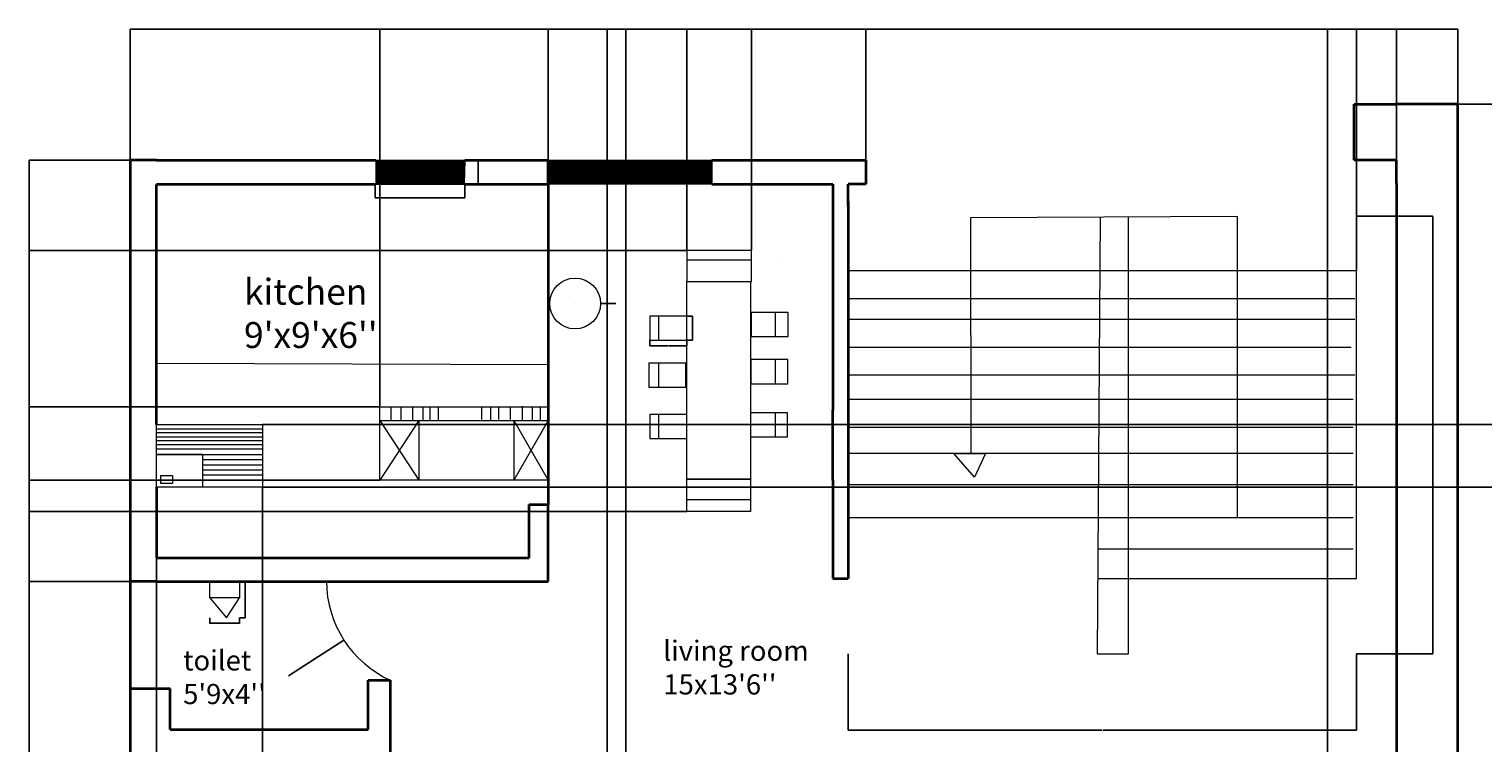
# Model space of a CAD drawing. Units: millimetres. Extents: x 1942 to 12281, y -2698 to 3078.
# Tile 3 of 6: x 1942 to 6981, y 552 to 3026. Entities that reach past the tile are written whole.
import ezdxf

# ---------------------------------------------------------------- set-up
doc = ezdxf.new("R2010")
doc.units = ezdxf.units.MM
for name, color, linetype, lineweight in [('A-ANNO-DIMS', 2, 'Continuous', 18), ('A-AREA-IDEN', 3, 'Continuous', 18), ('A-DETL-REF', 8, 'Continuous', 13), ('A-DOOR', 4, 'Continuous', 18), ('A-FLOR-FIXT', 9, 'Continuous', 18), ('A-FLOR-STRS', 7, 'Continuous', 18), ('A-FURN', 8, 'Continuous', 18), ('A-GLAZ', 4, 'Continuous', 18), ('A-GLAZ-PATT', 9, 'Continuous', 13), ('A-WALL', 7, 'Continuous', 35)]:
    doc.layers.add(name, color=color, linetype=linetype, lineweight=lineweight)
doc.styles.get("Standard").update_dxf_attribs({"font": 'arial.ttf'})
doc.dimstyles.get("Standard").update_dxf_attribs({"dimtxt": 0.18, "dimasz": 0.18, "dimexe": 0.18, "dimexo": 0.0625, "dimgap": 0.09, "dimtad": 0, "dimtih": 1, "dimtoh": 1, "dimdec": 4, "dimzin": 0, "dimdsep": 46, "dimtxsty": 'Standard', "dimcen": 0.09, "dimadec": 0, "dimazin": 0, "dimtfac": 1, "dimtdec": 4, "dimtofl": 0, "dimtmove": 0, "dimatfit": 3, "dimfxl": 1, "dimtolj": 1, "dimtzin": 0, "dimarcsym": 0})

# ---------------------------------------------------------------- blocks, each defined once
blk = doc.blocks.new('STAIR-RETURN')
for p, q in [((423.4, 1512.5), (1348.3, 1516.9)), ((423.4, 1512.5), (425.2, 695.6)), ((873.7, 1514.6), (863.4, 0)), ((972, 0), (972, 1515.1)), ((1348.3, 1516.9), (1348.3, 695.6)), ((0, 1328.6), (1761.6, 1328.6)), ((1761.6, 261.6), (1761.6, 1328.6)), ((0, 1232.1), (1755.6, 1232.1)), ((0, 1159.8), (1755.6, 1159.8)), ((0, 1063.3), (1743.5, 1063.3)), ((0, 966.9), (1755.6, 966.9)), ((0, 882.5), (1749.6, 882.5)), ((0, 786.1), (1749.6, 786.1)), ((0, 695.6), (1749.6, 695.6)), ((365.9, 694.8), (476.3, 694.8)), ((365.9, 694.8), (476.3, 694.8)), ((365.9, 694.8), (476.3, 694.8)), ((365.9, 694.8), (476.3, 694.8)), ((365.9, 694.8), (476.3, 694.8)), ((365.9, 694.8), (476.3, 694.8)), ((437.5, 612.8), (365.9, 694.8)), ((365.9, 694.8), (476.3, 694.8)), ((476.3, 694.8), (437.5, 612.8)), ((1348.3, 695.6), (1348.3, 587.1)), ((0, 587.1), (1749.6, 587.1)), ((1348.3, 587.1), (1348.3, 472.6)), ((0, 472.6), (1749.6, 472.6)), ((865.9, 364.1), (1749.6, 364.1)), ((865.2, 261.6), (1761.6, 261.6)), ((863.4, 0), (972, 0))]:
    blk.add_line(p, q)
blk = doc.blocks.new('WC-TAPERED')
for p, q in [((0, 69.7), (57.2, 0)), ((57.2, 0), (103.2, 69.7))]:
    blk.add_line(p, q)
blk.add_lwpolyline([(0, 126.7), (103.2, 126.7), (103.2, 69.7), (0, 69.7)], close=True)
blk = doc.blocks.new('DOOR-WC-LIVING')
blk.add_arc((380.4, 345.6), 380.4, 180.4328, 245.2749)
blk = doc.blocks.new('CHAIR-DINING')
blk.add_line((30.3, 83.7), (30.3, 0))
blk.add_lwpolyline([(128.3, 83.7), (0, 83.7), (0, 0), (128.3, 0)], close=True)
blk = doc.blocks.new('WIN-308')
for p, q in [((2.1, 83.8), (2.1, 0)), ((2.1, 83.8), (310.4, 83.8)), ((310.4, 83.8), (308.2, 0.3)), ((0, 0.3), (308.2, 0.3))]:
    blk.add_line(p, q)
blk = doc.blocks.new('WIN-567')
for p, q in [((0, 83.5), (0, 0)), ((0, 83.5), (567, 83.5)), ((567, 83.5), (567, 0)), ((567, 0), (0, 0))]:
    blk.add_line(p, q)
blk = doc.blocks.new('*D24')
at = {"layer": 'A-ANNO-DIMS', "color": 0, "lineweight": -2, "transparency": 16777216}
for p, q in [((4781.3, 860.5), (4781.3, 596.2)), ((6542.9, 860.5), (6542.9, 596.2)), ((4781.5, 596.4), (5660.5, 596.4)), ((6542.7, 596.4), (5663.7, 596.4))]:
    blk.add_line(p, q, dxfattribs=at)
at = {"layer": 'A-ANNO-DIMS', "color": 0, "transparency": 16777216}
for points in [[(4781.5, 596.4), (4781.5, 596.3), (4781.3, 596.4)], [(6542.7, 596.4), (6542.7, 596.3), (6542.9, 596.4)]]:
    blk.add_solid(points, dxfattribs=at)
at = {"layer": 'Defpoints', "color": 0, "transparency": 16777216}
for p in [(4781.3, 860.6), (6542.9, 860.6), (6542.9, 596.4)]:
    blk.add_point(p, dxfattribs=at)
at = {"layer": 'A-ANNO-DIMS', "color": 0, "transparency": 16777216, "insert": (5662.1, 596.4), "char_height": 0.18, "attachment_point": 5}
blk.add_mtext('\\A1;RETURN STAIR 1762 TYP.', dxfattribs=at)
blk = doc.blocks.new('*D25')
at = {"layer": 'A-ANNO-DIMS', "color": 0, "lineweight": -2, "transparency": 16777216}
for p, q in [((6543, 2377.5), (6807.4, 2377.5)), ((6807.2, 2377.3), (6807.2, 1619.2)), ((6807.2, 860.8), (6807.2, 1618.9)), ((6543, 860.6), (6807.4, 860.6))]:
    blk.add_line(p, q, dxfattribs=at)
at = {"layer": 'A-ANNO-DIMS', "color": 0, "transparency": 16777216}
for points in [[(6807.1, 2377.3), (6807.2, 2377.3), (6807.2, 2377.5)], [(6807.1, 860.8), (6807.2, 860.8), (6807.2, 860.6)]]:
    blk.add_solid(points, dxfattribs=at)
at = {"layer": 'Defpoints', "color": 0, "transparency": 16777216}
for p in [(6542.9, 2377.5), (6807.2, 2377.5), (6542.9, 860.6)]:
    blk.add_point(p, dxfattribs=at)
at = {"layer": 'A-ANNO-DIMS', "color": 0, "transparency": 16777216, "insert": (6807.2, 1619), "char_height": 0.18, "attachment_point": 5}
blk.add_mtext('\\A1;1517 TYP.', dxfattribs=at)
blk = doc.blocks.new('*D34')
at = {"layer": 'A-ANNO-DIMS', "color": 0, "lineweight": -2, "transparency": 16777216}
for p, q in [((2671.7, 1112.6), (2690.8, 1112.6)), ((2690.6, 1112.4), (2690.6, 1049.4)), ((2690.6, 986), (2690.6, 1049)), ((2671.7, 985.9), (2690.8, 985.9))]:
    blk.add_line(p, q, dxfattribs=at)
at = {"layer": 'A-ANNO-DIMS', "color": 0, "transparency": 16777216}
for points in [[(2690.6, 1112.4), (2690.7, 1112.4), (2690.6, 1112.6)], [(2690.6, 986), (2690.7, 986), (2690.6, 985.9)]]:
    blk.add_solid(points, dxfattribs=at)
at = {"layer": 'Defpoints', "color": 0, "transparency": 16777216}
for p in [(2671.6, 1112.6), (2690.6, 1112.6), (2671.6, 985.9)]:
    blk.add_point(p, dxfattribs=at)
at = {"layer": 'A-ANNO-DIMS', "color": 0, "transparency": 16777216, "insert": (2690.6, 1049.2), "char_height": 0.18, "attachment_point": 5}
blk.add_mtext('\\A1;WC 127 TYP.', dxfattribs=at)
blk = doc.blocks.new('*D35')
at = {"layer": 'A-ANNO-DIMS', "color": 0, "lineweight": -2, "transparency": 16777216}
for p, q in [((2568.4, 985.8), (2568.4, 966.7)), ((2568.6, 966.9), (2619.4, 966.9)), ((2671.5, 966.9), (2620.6, 966.9)), ((2671.6, 985.8), (2671.6, 966.7))]:
    blk.add_line(p, q, dxfattribs=at)
at = {"layer": 'A-ANNO-DIMS', "color": 0, "transparency": 16777216}
for points in [[(2568.6, 966.9), (2568.6, 966.8), (2568.4, 966.9)], [(2671.5, 966.9), (2671.5, 966.8), (2671.6, 966.9)]]:
    blk.add_solid(points, dxfattribs=at)
at = {"layer": 'Defpoints', "color": 0, "transparency": 16777216}
for p in [(2568.4, 985.9), (2671.6, 985.9), (2671.6, 966.9)]:
    blk.add_point(p, dxfattribs=at)
at = {"layer": 'A-ANNO-DIMS', "color": 0, "transparency": 16777216, "insert": (2620, 966.9), "char_height": 0.18, "attachment_point": 5}
blk.add_mtext('\\A1;103 TYP.', dxfattribs=at)
blk = doc.blocks.new('*D46')
at = {"layer": 'A-ANNO-DIMS', "color": 0, "lineweight": -2, "transparency": 16777216}
for p, q in [((4093.4, 1948), (4093.4, 1928.6)), ((4093.6, 1928.8), (4156.5, 1928.8)), ((4221.5, 1928.8), (4158.5, 1928.8)), ((4221.6, 1948), (4221.6, 1928.6))]:
    blk.add_line(p, q, dxfattribs=at)
at = {"layer": 'A-ANNO-DIMS', "color": 0, "transparency": 16777216}
for points in [[(4093.6, 1928.9), (4093.6, 1928.8), (4093.4, 1928.8)], [(4221.5, 1928.9), (4221.5, 1928.8), (4221.6, 1928.8)]]:
    blk.add_solid(points, dxfattribs=at)
at = {"layer": 'Defpoints', "color": 0, "transparency": 16777216}
for p in [(4093.4, 1948.1), (4221.6, 1948.1), (4221.6, 1928.8)]:
    blk.add_point(p, dxfattribs=at)
at = {"layer": 'A-ANNO-DIMS', "color": 0, "transparency": 16777216, "insert": (4157.5, 1928.8), "char_height": 0.18, "attachment_point": 5}
blk.add_mtext('\\A1;CHAIR 128 TYP.', dxfattribs=at)
blk = doc.blocks.new('*D47')
at = {"layer": 'A-ANNO-DIMS', "color": 0, "lineweight": -2, "transparency": 16777216}
for p, q in [((4221.7, 2031.8), (4241.1, 2031.8)), ((4240.9, 2031.6), (4240.9, 1990.1)), ((4240.9, 1948.2), (4240.9, 1989.7)), ((4221.7, 1948.1), (4241.1, 1948.1))]:
    blk.add_line(p, q, dxfattribs=at)
at = {"layer": 'A-ANNO-DIMS', "color": 0, "transparency": 16777216}
for points in [[(4240.8, 2031.6), (4240.9, 2031.6), (4240.9, 2031.8)], [(4240.8, 1948.2), (4240.9, 1948.2), (4240.9, 1948.1)]]:
    blk.add_solid(points, dxfattribs=at)
at = {"layer": 'Defpoints', "color": 0, "transparency": 16777216}
for p in [(4221.6, 2031.8), (4240.9, 2031.8), (4221.6, 1948.1)]:
    blk.add_point(p, dxfattribs=at)
at = {"layer": 'A-ANNO-DIMS', "color": 0, "transparency": 16777216, "insert": (4240.9, 1989.9), "char_height": 0.18, "attachment_point": 5}
blk.add_mtext('\\A1;84 TYP.', dxfattribs=at)
blk = doc.blocks.new('*D60')
at = {"layer": 'A-ANNO-DIMS', "color": 0, "lineweight": -2, "transparency": 16777216}
for p, q in [((3141.6, 2488.1), (3141.6, 2441.4)), ((3452, 2488.1), (3452, 2441.4)), ((3141.8, 2441.6), (3296, 2441.6)), ((3451.8, 2441.6), (3297.7, 2441.6))]:
    blk.add_line(p, q, dxfattribs=at)
at = {"layer": 'A-ANNO-DIMS', "color": 0, "transparency": 16777216}
for points in [[(3141.8, 2441.6), (3141.8, 2441.6), (3141.6, 2441.6)], [(3451.8, 2441.6), (3451.8, 2441.6), (3452, 2441.6)]]:
    blk.add_solid(points, dxfattribs=at)
at = {"layer": 'Defpoints', "color": 0, "transparency": 16777216}
for p in [(3141.6, 2488.2), (3452, 2488.2), (3452, 2441.6)]:
    blk.add_point(p, dxfattribs=at)
at = {"layer": 'A-ANNO-DIMS', "color": 0, "transparency": 16777216, "insert": (3296.8, 2441.6), "char_height": 0.18, "attachment_point": 5}
blk.add_mtext('\\A1;W1 310 TYP.', dxfattribs=at)
blk = doc.blocks.new('*D61')
at = {"layer": 'A-ANNO-DIMS', "color": 0, "lineweight": -2, "transparency": 16777216}
for p, q in [((3452.1, 2572), (3498.8, 2572)), ((3498.6, 2571.8), (3498.6, 2530.2)), ((3498.6, 2488.3), (3498.6, 2529.9)), ((3452.1, 2488.2), (3498.8, 2488.2))]:
    blk.add_line(p, q, dxfattribs=at)
at = {"layer": 'A-ANNO-DIMS', "color": 0, "transparency": 16777216}
for points in [[(3498.6, 2571.8), (3498.6, 2571.8), (3498.6, 2572)], [(3498.6, 2488.3), (3498.6, 2488.3), (3498.6, 2488.2)]]:
    blk.add_solid(points, dxfattribs=at)
at = {"layer": 'Defpoints', "color": 0, "transparency": 16777216}
for p in [(3452, 2572), (3498.6, 2572), (3452, 2488.2)]:
    blk.add_point(p, dxfattribs=at)
at = {"layer": 'A-ANNO-DIMS', "color": 0, "transparency": 16777216, "insert": (3498.6, 2530.1), "char_height": 0.18, "attachment_point": 5}
blk.add_mtext('\\A1;84 TYP.', dxfattribs=at)
blk = doc.blocks.new('*D70')
at = {"layer": 'A-ANNO-DIMS', "color": 0, "lineweight": -2, "transparency": 16777216}
for p, q in [((2292.1, 2572), (2292.1, 3026.3)), ((2292.2, 3026.1), (4592.7, 3026.1)), ((6893.9, 3026.1), (4593.4, 3026.1)), ((6894.1, 2765.9), (6894.1, 3026.3))]:
    blk.add_line(p, q, dxfattribs=at)
at = {"layer": 'A-ANNO-DIMS', "color": 0, "transparency": 16777216}
for points in [[(2292.2, 3026.2), (2292.2, 3026.1), (2292.1, 3026.1)], [(6893.9, 3026.2), (6893.9, 3026.1), (6894.1, 3026.1)]]:
    blk.add_solid(points, dxfattribs=at)
at = {"layer": 'Defpoints', "color": 0, "transparency": 16777216}
for p in [(6894.1, 3026.1), (6894.1, 2765.9), (2292.1, 2572)]:
    blk.add_point(p, dxfattribs=at)
at = {"layer": 'A-ANNO-DIMS', "color": 0, "transparency": 16777216, "insert": (4593.1, 3026.1), "char_height": 0.18, "attachment_point": 5}
blk.add_mtext('\\A1;4602', dxfattribs=at)
blk = doc.blocks.new('*D71')
at = {"layer": 'A-ANNO-DIMS', "color": 0, "lineweight": -2, "transparency": 16777216}
for p, q in [((6894.2, 2765.9), (7154.5, 2765.9)), ((7154.3, 2765.7), (7154.3, 164.5)), ((7154.3, -2437.1), (7154.3, 164.1)), ((6894.2, -2437.2), (7154.5, -2437.2))]:
    blk.add_line(p, q, dxfattribs=at)
at = {"layer": 'A-ANNO-DIMS', "color": 0, "transparency": 16777216}
for points in [[(7154.3, 2765.7), (7154.4, 2765.7), (7154.3, 2765.9)], [(7154.3, -2437.1), (7154.4, -2437.1), (7154.3, -2437.2)]]:
    blk.add_solid(points, dxfattribs=at)
at = {"layer": 'Defpoints', "color": 0, "transparency": 16777216}
for p in [(6894.1, 2765.9), (7154.3, 2765.9), (6894.1, -2437.2)]:
    blk.add_point(p, dxfattribs=at)
at = {"layer": 'A-ANNO-DIMS', "color": 0, "transparency": 16777216, "insert": (7154.3, 164.3), "char_height": 0.18, "attachment_point": 5}
blk.add_mtext('\\A1;5203', dxfattribs=at)
blk = doc.blocks.new('*D74')
at = {"layer": 'A-ANNO-DIMS', "color": 0, "lineweight": -2, "transparency": 16777216}
for p, q in [((2292.1, 2572), (2292.1, 3026.3)), ((2292.2, 3026.1), (3016.3, 3026.1)), ((3741.2, 3026.1), (3017.2, 3026.1)), ((3741.4, 2572), (3741.4, 3026.3))]:
    blk.add_line(p, q, dxfattribs=at)
at = {"layer": 'A-ANNO-DIMS', "color": 0, "transparency": 16777216}
for points in [[(2292.2, 3026.2), (2292.2, 3026.1), (2292.1, 3026.1)], [(3741.2, 3026.2), (3741.2, 3026.1), (3741.4, 3026.1)]]:
    blk.add_solid(points, dxfattribs=at)
at = {"layer": 'Defpoints', "color": 0, "transparency": 16777216}
for p in [(3741.4, 3026.1), (2292.1, 2572), (3741.4, 2572)]:
    blk.add_point(p, dxfattribs=at)
at = {"layer": 'A-ANNO-DIMS', "color": 0, "transparency": 16777216, "insert": (3016.7, 3026.1), "char_height": 0.18, "attachment_point": 5}
blk.add_mtext('\\A1;1449.3', dxfattribs=at)
blk = doc.blocks.new('*D75')
at = {"layer": 'A-ANNO-DIMS', "color": 0, "lineweight": -2, "transparency": 16777216}
for p, q in [((3741.4, 2572), (3741.4, 3026.3)), ((3741.6, 3026.1), (4291.5, 3026.1)), ((4842.4, 3026.1), (4292.4, 3026.1)), ((4842.6, 2572), (4842.6, 3026.3))]:
    blk.add_line(p, q, dxfattribs=at)
at = {"layer": 'A-ANNO-DIMS', "color": 0, "transparency": 16777216}
for points in [[(3741.6, 3026.2), (3741.6, 3026.1), (3741.4, 3026.1)], [(4842.4, 3026.2), (4842.4, 3026.1), (4842.6, 3026.1)]]:
    blk.add_solid(points, dxfattribs=at)
at = {"layer": 'Defpoints', "color": 0, "transparency": 16777216}
for p in [(4842.6, 3026.1), (3741.4, 2572), (4842.6, 2572)]:
    blk.add_point(p, dxfattribs=at)
at = {"layer": 'A-ANNO-DIMS', "color": 0, "transparency": 16777216, "insert": (4292, 3026.1), "char_height": 0.18, "attachment_point": 5}
blk.add_mtext('\\A1;1101.2', dxfattribs=at)
blk = doc.blocks.new('*D76')
at = {"layer": 'A-ANNO-DIMS', "color": 0, "lineweight": -2, "transparency": 16777216}
for p, q in [((2292, 2572), (1942, 2572)), ((1942.2, 2571.8), (1942.2, 1842.2)), ((1942.2, 1112.2), (1942.2, 1841.8)), ((2292, 1112.1), (1942, 1112.1))]:
    blk.add_line(p, q, dxfattribs=at)
at = {"layer": 'A-ANNO-DIMS', "color": 0, "transparency": 16777216}
for points in [[(1942.2, 2571.8), (1942.2, 2571.8), (1942.2, 2572)], [(1942.2, 1112.2), (1942.2, 1112.2), (1942.2, 1112.1)]]:
    blk.add_solid(points, dxfattribs=at)
at = {"layer": 'Defpoints', "color": 0, "transparency": 16777216}
for p in [(1942.2, 2572), (2292.1, 2572), (2292.1, 1112.1)]:
    blk.add_point(p, dxfattribs=at)
at = {"layer": 'A-ANNO-DIMS', "color": 0, "transparency": 16777216, "insert": (1942.2, 1842), "char_height": 0.18, "attachment_point": 5}
blk.add_mtext('\\A1;1460', dxfattribs=at)
blk = doc.blocks.new('*D77')
at = {"layer": 'A-ANNO-DIMS', "color": 0, "lineweight": -2, "transparency": 16777216}
for p, q in [((2292, 1112.1), (1942, 1112.1)), ((1942.2, 1111.9), (1942.2, 802.3)), ((1942.2, 492.4), (1942.2, 801.9)), ((3116.8, 492.2), (1942, 492.2))]:
    blk.add_line(p, q, dxfattribs=at)
at = {"layer": 'A-ANNO-DIMS', "color": 0, "transparency": 16777216}
for points in [[(1942.2, 1111.9), (1942.2, 1111.9), (1942.2, 1112.1)], [(1942.2, 492.4), (1942.2, 492.4), (1942.2, 492.2)]]:
    blk.add_solid(points, dxfattribs=at)
at = {"layer": 'Defpoints', "color": 0, "transparency": 16777216}
for p in [(1942.2, 1112.1), (2292.1, 1112.1), (3116.8, 492.2)]:
    blk.add_point(p, dxfattribs=at)
at = {"layer": 'A-ANNO-DIMS', "color": 0, "transparency": 16777216, "insert": (1942.2, 802.1), "char_height": 0.18, "attachment_point": 5}
blk.add_mtext('\\A1;619.9', dxfattribs=at)
blk = doc.blocks.new('*D80')
at = {"layer": 'A-ANNO-DIMS', "color": 0, "lineweight": -2, "transparency": 16777216}
for p, q in [((2292.1, 1112), (2292.1, -2697.7)), ((3193.8, 769.3), (3193.8, -2697.7)), ((2292.2, -2697.5), (2742.5, -2697.5)), ((3193.6, -2697.5), (2743.3, -2697.5))]:
    blk.add_line(p, q, dxfattribs=at)
at = {"layer": 'A-ANNO-DIMS', "color": 0, "transparency": 16777216}
for points in [[(2292.2, -2697.5), (2292.2, -2697.5), (2292.1, -2697.5)], [(3193.6, -2697.5), (3193.6, -2697.5), (3193.8, -2697.5)]]:
    blk.add_solid(points, dxfattribs=at)
at = {"layer": 'Defpoints', "color": 0, "transparency": 16777216}
for p in [(2292.1, 1112.1), (3193.8, 769.4), (3193.8, -2697.5)]:
    blk.add_point(p, dxfattribs=at)
at = {"layer": 'A-ANNO-DIMS', "color": 0, "transparency": 16777216, "insert": (2742.9, -2697.5), "char_height": 0.18, "attachment_point": 5}
blk.add_mtext('\\A1;901.7', dxfattribs=at)
blk = doc.blocks.new('*D82')
at = {"layer": 'A-ANNO-DIMS', "color": 0, "lineweight": -2, "transparency": 16777216}
for p, q in [((6442.7, -769.4), (6442.7, 3026.3)), ((6442.9, 3026.1), (6561.6, 3026.1)), ((6681.3, 3026.1), (6562.6, 3026.1)), ((6681.5, -769.5), (6681.5, 3026.3))]:
    blk.add_line(p, q, dxfattribs=at)
at = {"layer": 'A-ANNO-DIMS', "color": 0, "transparency": 16777216}
for points in [[(6442.9, 3026.2), (6442.9, 3026.1), (6442.7, 3026.1)], [(6681.3, 3026.2), (6681.3, 3026.1), (6681.5, 3026.1)]]:
    blk.add_solid(points, dxfattribs=at)
at = {"layer": 'Defpoints', "color": 0, "transparency": 16777216}
for p in [(6681.5, 3026.1), (6442.7, -769.5), (6681.5, -769.5)]:
    blk.add_point(p, dxfattribs=at)
at = {"layer": 'A-ANNO-DIMS', "color": 0, "transparency": 16777216, "insert": (6562.1, 3026.1), "char_height": 0.18, "attachment_point": 5}
blk.add_mtext('\\A1;238.74', dxfattribs=at)
blk = doc.blocks.new('*D83')
at = {"layer": 'A-ANNO-DIMS', "color": 0, "lineweight": -2, "transparency": 16777216}
for p, q in [((4221.6, 2259.5), (4221.6, 3026.3)), ((4221.8, 3026.1), (4333.4, 3026.1)), ((4446, 3026.1), (4334.4, 3026.1)), ((4446.2, 2259.5), (4446.2, 3026.3))]:
    blk.add_line(p, q, dxfattribs=at)
at = {"layer": 'A-ANNO-DIMS', "color": 0, "transparency": 16777216}
for points in [[(4221.8, 3026.2), (4221.8, 3026.1), (4221.6, 3026.1)], [(4446, 3026.2), (4446, 3026.1), (4446.2, 3026.1)]]:
    blk.add_solid(points, dxfattribs=at)
at = {"layer": 'Defpoints', "color": 0, "transparency": 16777216}
for p in [(4446.2, 3026.1), (4221.6, 2259.4), (4446.2, 2259.4)]:
    blk.add_point(p, dxfattribs=at)
at = {"layer": 'A-ANNO-DIMS', "color": 0, "transparency": 16777216, "insert": (4333.9, 3026.1), "char_height": 0.18, "attachment_point": 5}
blk.add_mtext('\\A1;224.52', dxfattribs=at)
blk = doc.blocks.new('*D84')
at = {"layer": 'A-ANNO-DIMS', "color": 0, "lineweight": -2, "transparency": 16777216}
for p, q in [((4221.6, 2259.4), (1942, 2259.4)), ((1942.2, 2259.3), (1942.2, 1807)), ((1942.2, 1354.5), (1942.2, 1806.7)), ((4221.6, 1354.3), (1942, 1354.3))]:
    blk.add_line(p, q, dxfattribs=at)
at = {"layer": 'A-ANNO-DIMS', "color": 0, "transparency": 16777216}
for points in [[(1942.2, 2259.3), (1942.2, 2259.3), (1942.2, 2259.4)], [(1942.2, 1354.5), (1942.2, 1354.5), (1942.2, 1354.3)]]:
    blk.add_solid(points, dxfattribs=at)
at = {"layer": 'Defpoints', "color": 0, "transparency": 16777216}
for p in [(1942.2, 2259.4), (4221.6, 2259.4), (4221.6, 1354.3)]:
    blk.add_point(p, dxfattribs=at)
at = {"layer": 'A-ANNO-DIMS', "color": 0, "transparency": 16777216, "insert": (1942.2, 1806.9), "char_height": 0.18, "attachment_point": 5}
blk.add_mtext('\\A1;905.2', dxfattribs=at)
blk = doc.blocks.new('*D85')
at = {"layer": 'A-ANNO-DIMS', "color": 0, "lineweight": -2, "transparency": 16777216}
for p, q in [((2384.1, 1439.1), (2384.1, -2697.7)), ((2750.5, 1439.1), (2750.5, -2697.7)), ((2384.3, -2697.5), (2566.9, -2697.5)), ((2750.3, -2697.5), (2567.7, -2697.5))]:
    blk.add_line(p, q, dxfattribs=at)
at = {"layer": 'A-ANNO-DIMS', "color": 0, "transparency": 16777216}
for points in [[(2384.3, -2697.5), (2384.3, -2697.5), (2384.1, -2697.5)], [(2750.3, -2697.5), (2750.3, -2697.5), (2750.5, -2697.5)]]:
    blk.add_solid(points, dxfattribs=at)
at = {"layer": 'Defpoints', "color": 0, "transparency": 16777216}
for p in [(2384.1, 1439.2), (2750.5, 1439.2), (2750.5, -2697.5)]:
    blk.add_point(p, dxfattribs=at)
at = {"layer": 'A-ANNO-DIMS', "color": 0, "transparency": 16777216, "insert": (2567.3, -2697.5), "char_height": 0.18, "attachment_point": 5}
blk.add_mtext('\\A1;366.4', dxfattribs=at)
blk = doc.blocks.new('*D86')
at = {"layer": 'A-ANNO-DIMS', "color": 0, "lineweight": -2, "transparency": 16777216}
for p, q in [((2750.6, 1655.8), (7154.5, 1655.8)), ((7154.3, 1655.6), (7154.3, 1547.7)), ((7154.3, 1439.4), (7154.3, 1547.3)), ((2750.6, 1439.2), (7154.5, 1439.2))]:
    blk.add_line(p, q, dxfattribs=at)
at = {"layer": 'A-ANNO-DIMS', "color": 0, "transparency": 16777216}
for points in [[(7154.3, 1655.6), (7154.4, 1655.6), (7154.3, 1655.8)], [(7154.3, 1439.4), (7154.4, 1439.4), (7154.3, 1439.2)]]:
    blk.add_solid(points, dxfattribs=at)
at = {"layer": 'Defpoints', "color": 0, "transparency": 16777216}
for p in [(2750.5, 1655.8), (7154.3, 1655.8), (2750.5, 1439.2)]:
    blk.add_point(p, dxfattribs=at)
at = {"layer": 'A-ANNO-DIMS', "color": 0, "transparency": 16777216, "insert": (7154.3, 1547.5), "char_height": 0.18, "attachment_point": 5}
blk.add_mtext('\\A1;216.57', dxfattribs=at)
blk = doc.blocks.new('*D87')
at = {"layer": 'A-ANNO-DIMS', "color": 0, "lineweight": -2, "transparency": 16777216}
for p, q in [((3158, 1717.7), (3158, 3026.3)), ((3158.1, 3026.1), (3449.3, 3026.1)), ((3741.2, 3026.1), (3450.1, 3026.1)), ((3741.4, 1717.7), (3741.4, 3026.3))]:
    blk.add_line(p, q, dxfattribs=at)
at = {"layer": 'A-ANNO-DIMS', "color": 0, "transparency": 16777216}
for points in [[(3158.1, 3026.2), (3158.1, 3026.1), (3158, 3026.1)], [(3741.2, 3026.2), (3741.2, 3026.1), (3741.4, 3026.1)]]:
    blk.add_solid(points, dxfattribs=at)
at = {"layer": 'Defpoints', "color": 0, "transparency": 16777216}
for p in [(3741.4, 3026.1), (3158, 1717.6), (3741.4, 1717.6)]:
    blk.add_point(p, dxfattribs=at)
at = {"layer": 'A-ANNO-DIMS', "color": 0, "transparency": 16777216, "insert": (3449.7, 3026.1), "char_height": 0.18, "attachment_point": 5}
blk.add_mtext('\\A1;583.4', dxfattribs=at)
blk = doc.blocks.new('*D88')
at = {"layer": 'A-ANNO-DIMS', "color": 0, "lineweight": -2, "transparency": 16777216}
for p, q in [((3157.9, 1717.6), (1942, 1717.6)), ((1942.2, 1717.4), (1942.2, 1590.7)), ((1942.2, 1463.7), (1942.2, 1590.4)), ((3157.9, 1463.5), (1942, 1463.5))]:
    blk.add_line(p, q, dxfattribs=at)
at = {"layer": 'A-ANNO-DIMS', "color": 0, "transparency": 16777216}
for points in [[(1942.2, 1717.4), (1942.2, 1717.4), (1942.2, 1717.6)], [(1942.2, 1463.7), (1942.2, 1463.7), (1942.2, 1463.5)]]:
    blk.add_solid(points, dxfattribs=at)
at = {"layer": 'Defpoints', "color": 0, "transparency": 16777216}
for p in [(1942.2, 1717.6), (3158, 1717.6), (3158, 1463.5)]:
    blk.add_point(p, dxfattribs=at)
at = {"layer": 'A-ANNO-DIMS', "color": 0, "transparency": 16777216, "insert": (1942.2, 1590.5), "char_height": 0.18, "attachment_point": 5}
blk.add_mtext('\\A1;254.1', dxfattribs=at)
blk = doc.blocks.new('*D89')
at = {"layer": 'A-ANNO-DIMS', "color": 0, "lineweight": -2, "transparency": 16777216}
for p, q in [((3945.3, -2351.5), (3945.3, 3026.3)), ((3945.5, 3026.1), (3977.7, 3026.1)), ((4010.5, 3026.1), (3978.3, 3026.1)), ((4010.7, -2351.5), (4010.7, 3026.3))]:
    blk.add_line(p, q, dxfattribs=at)
at = {"layer": 'A-ANNO-DIMS', "color": 0, "transparency": 16777216}
for points in [[(3945.5, 3026.2), (3945.5, 3026.1), (3945.3, 3026.1)], [(4010.5, 3026.2), (4010.5, 3026.1), (4010.7, 3026.1)]]:
    blk.add_solid(points, dxfattribs=at)
at = {"layer": 'Defpoints', "color": 0, "transparency": 16777216}
for p in [(4010.7, 3026.1), (3945.3, -2351.6), (4010.7, -2351.6)]:
    blk.add_point(p, dxfattribs=at)
at = {"layer": 'A-ANNO-DIMS', "color": 0, "transparency": 16777216, "insert": (3978, 3026.1), "char_height": 0.18, "attachment_point": 5}
blk.add_mtext('\\A1;65.4', dxfattribs=at)
blk = doc.blocks.new('*D90')
at = {"layer": 'A-ANNO-DIMS', "color": 0, "lineweight": -2, "transparency": 16777216}
for p, q in [((6681.5, -2351.5), (6681.5, 3026.3)), ((6681.6, 3026.1), (6787.3, 3026.1)), ((6893.9, 3026.1), (6788.2, 3026.1)), ((6894.1, -2437.2), (6894.1, 3026.3))]:
    blk.add_line(p, q, dxfattribs=at)
at = {"layer": 'A-ANNO-DIMS', "color": 0, "transparency": 16777216}
for points in [[(6681.6, 3026.2), (6681.6, 3026.1), (6681.5, 3026.1)], [(6893.9, 3026.2), (6893.9, 3026.1), (6894.1, 3026.1)]]:
    blk.add_solid(points, dxfattribs=at)
at = {"layer": 'Defpoints', "color": 0, "transparency": 16777216}
for p in [(6894.1, 3026.1), (6681.5, -2351.6), (6894.1, -2437.2)]:
    blk.add_point(p, dxfattribs=at)
at = {"layer": 'A-ANNO-DIMS', "color": 0, "transparency": 16777216, "insert": (6787.8, 3026.1), "char_height": 0.18, "attachment_point": 5}
blk.add_mtext('\\A1;212.64', dxfattribs=at)
blk = doc.blocks.new('*D91')
at = {"layer": 'A-ANNO-DIMS', "color": 0, "lineweight": -2, "transparency": 16777216}
for p, q in [((6542.9, 2189.3), (6542.9, 3026.3)), ((6543.1, 3026.1), (6611.7, 3026.1)), ((6681.3, 3026.1), (6612.6, 3026.1)), ((6681.5, 2572), (6681.5, 3026.3))]:
    blk.add_line(p, q, dxfattribs=at)
at = {"layer": 'A-ANNO-DIMS', "color": 0, "transparency": 16777216}
for points in [[(6543.1, 3026.2), (6543.1, 3026.1), (6542.9, 3026.1)], [(6681.3, 3026.2), (6681.3, 3026.1), (6681.5, 3026.1)]]:
    blk.add_solid(points, dxfattribs=at)
at = {"layer": 'Defpoints', "color": 0, "transparency": 16777216}
for p in [(6681.5, 3026.1), (6681.5, 2572), (6542.9, 2189.2)]:
    blk.add_point(p, dxfattribs=at)
at = {"layer": 'A-ANNO-DIMS', "color": 0, "transparency": 16777216, "insert": (6612.2, 3026.1), "char_height": 0.18, "attachment_point": 5}
blk.add_mtext('\\A1;138.53', dxfattribs=at)
blk = doc.blocks.new('*D117')
at = {"layer": 'A-ANNO-DIMS', "color": 0, "lineweight": -2, "transparency": 16777216}
for p, q in [((3352.8, 1114.9), (3353, 1114.9)), ((3352.9, 1114.8), (3352.9, 1115)), ((2841.5, 784.7), (3033.1, 908.5)), ((2841.4, 784.7), (2841.5, 784.7))]:
    blk.add_line(p, q, dxfattribs=at)
at = {"layer": 'A-ANNO-DIMS', "color": 0, "transparency": 16777216}
blk.add_solid([(3033.1, 908.5), (3033.2, 908.4), (3033.3, 908.5)], dxfattribs=at)
at = {"layer": 'Defpoints', "color": 0, "transparency": 16777216}
for p in [(3352.9, 1114.9), (3033.3, 908.5)]:
    blk.add_point(p, dxfattribs=at)
at = {"layer": 'A-ANNO-DIMS', "color": 0, "transparency": 16777216, "insert": (2840.6, 784.7), "char_height": 0.18, "attachment_point": 5}
blk.add_mtext('\\A1;2X R380.44', dxfattribs=at)
blk = doc.blocks.new('*D119')
at = {"layer": 'A-ANNO-DIMS', "color": 0, "lineweight": -2, "transparency": 16777216}
for p, q in [((3834.4, 2075.2), (3834.6, 2075.2)), ((3834.5, 2075.1), (3834.5, 2075.2)), ((3975.6, 2075.2), (3922.9, 2075.2))]:
    blk.add_line(p, q, dxfattribs=at)
at = {"layer": 'A-ANNO-DIMS', "color": 0, "transparency": 16777216}
blk.add_solid([(3922.9, 2075.2), (3922.9, 2075.1), (3922.7, 2075.2)], dxfattribs=at)
at = {"layer": 'Defpoints', "color": 0, "transparency": 16777216}
for p in [(3746.4, 2075.2), (3922.7, 2075.2)]:
    blk.add_point(p, dxfattribs=at)
at = {"layer": 'A-ANNO-DIMS', "color": 0, "transparency": 16777216, "insert": (3976.1, 2075.2), "char_height": 0.18, "attachment_point": 5}
blk.add_mtext('\\A1;∅176.3', dxfattribs=at)

msp = doc.modelspace()

# ---------------------------------------------------------------- hatches: boundary and pattern name
at = {"layer": 'A-GLAZ-PATT'}
h = msp.add_hatch(dxfattribs=at)
h.set_pattern_fill('ANSI31', color=256, scale=1.19991, angle=135, style=0)
h.paths.add_polyline_path([(3143.773, 2488.153), (3449.878, 2488.434), (3452.022, 2571.966), (3143.773, 2571.966)])
h = msp.add_hatch(dxfattribs=at)
h.set_pattern_fill('ANSI31', color=256, scale=1.384708, angle=135, style=0)
h.paths.add_polyline_path([(3741.389, 2488.434), (4308.364, 2488.434), (4308.364, 2571.966), (3741.389, 2571.966)])

# ---------------------------------------------------------------- linework, layer by layer
at = {"layer": 'A-DETL-REF'}
msp.add_line((4554.226, 2226.418), (4554.226, 2226.418), dxfattribs=at)
at = {"layer": 'A-FLOR-FIXT'}
for p, q in [((2384.129, 1868.242), (3741.389, 1863.301)), ((3157.957, 1669.733), (3157.957, 1717.597)), ((3157.957, 1717.597), (3741.389, 1717.597)), ((3196.752, 1670.413), (3196.752, 1718.277)), ((3232.144, 1669.733), (3232.144, 1717.597)), ((3271.959, 1670.073), (3271.959, 1717.937)), ((3307.692, 1669.393), (3307.692, 1717.257)), ((3331.844, 1670.263), (3331.844, 1718.128)), ((3361.46, 1669.393), (3361.46, 1717.257)), ((3511.007, 1673.209), (3511.007, 1717.597)), ((3542.642, 1672.004), (3542.642, 1717.597)), ((3570.35, 1673.209), (3570.35, 1717.597)), ((3610.585, 1673.209), (3610.585, 1717.597)), ((3652.397, 1671.133), (3652.397, 1718.998)), ((3686.368, 1668.522), (3686.368, 1716.387)), ((3714.243, 1668.522), (3714.243, 1716.387)), ((3741.389, 1717.597), (3741.061, 1669.733)), ((3293.444, 1669.733), (3157.957, 1463.478)), ((3157.957, 1669.733), (3293.444, 1463.478)), ((3293.444, 1669.733), (3293.444, 1463.478)), ((3622.376, 1669.733), (3622.376, 1463.478)), ((3622.376, 1669.733), (3741.061, 1463.478)), ((3741.061, 1669.733), (3622.376, 1463.478)), ((2384.129, 1640.901), (2750.504, 1640.901)), ((2384.129, 1627.614), (2750.504, 1627.614)), ((2384.129, 1613.441), (2750.504, 1613.441)), ((2383.243, 1586.867), (2750.504, 1586.867)), ((2384.129, 1600.154), (2750.504, 1600.154)), ((2384.129, 1571.808), (2750.504, 1571.808)), ((2384.129, 1553.212), (2542.946, 1553.212)), ((2385.016, 1552.32), (2750.504, 1552.32)), ((2542.806, 1534.604), (2750.504, 1534.604)), ((2542.946, 1553.212), (2542.946, 1439.211)), ((2543.693, 1516.003), (2750.504, 1516.003)), ((2544.579, 1498.287), (2750.504, 1498.287)), ((2545.466, 1481.456), (2750.504, 1481.456)), ((2549.012, 1463.74), (2750.504, 1463.74))]:
    msp.add_line(p, q, dxfattribs=at)
for points in [[(3157.957, 1669.733), (3741.061, 1669.733), (3741.061, 1463.478), (3157.957, 1463.478)], [(2384.129, 1655.778), (2750.504, 1655.778), (2750.504, 1439.211), (2384.129, 1439.211)], [(2398.569, 1478.645), (2438.779, 1478.645), (2438.779, 1451.481), (2398.569, 1451.481)]]:
    msp.add_lwpolyline(points, close=True, dxfattribs=at)
at = {"layer": 'A-FURN'}
for p, q in [((4221.636, 2226.418), (4446.16, 2226.418)), ((4528.176, 2044.398), (4528.176, 1960.672)), ((4123.635, 1868.904), (4123.635, 1785.178)), ((4528.176, 1881.082), (4528.176, 1797.356)), ((4528.176, 1696.885), (4528.176, 1613.159)), ((4221.636, 1395.707), (4442.289, 1395.707))]:
    msp.add_line(p, q, dxfattribs=at)
for points in [[(4221.636, 2151.138), (4446.16, 2151.138), (4446.16, 2259.448), (4221.636, 2259.448)], [(4221.636, 2151.138), (4442.289, 2151.138), (4442.289, 1466.465), (4221.636, 1466.465)], [(4573.532, 2044.398), (4445.272, 2044.398), (4445.272, 1960.672), (4573.532, 1960.672)], [(4218.589, 1868.904), (4090.329, 1868.904), (4090.329, 1785.178), (4218.589, 1785.178)], [(4572.024, 1881.082), (4443.764, 1881.082), (4443.764, 1797.356), (4572.024, 1797.356)], [(4570.501, 1696.885), (4442.241, 1696.885), (4442.241, 1613.159), (4570.501, 1613.159)], [(4221.636, 1466.465), (4442.289, 1466.465), (4442.289, 1354.287), (4221.636, 1354.287)]]:
    msp.add_lwpolyline(points, close=True, dxfattribs=at)
msp.add_circle((3834.527, 2075.157), 88.151, dxfattribs=at)
at = {"layer": 'A-WALL'}
for p, q in [((6534.554, 2571.966), (6534.554, 2765.873)), ((6534.554, 2765.873), (6678.321, 2765.873)), ((6894.096, 2765.873), (6678.321, 2765.873)), ((6894.096, -486.223), (6894.096, 2765.873)), ((2384.129, 2571.966), (2292.051, 2571.966)), ((2292.051, 2571.966), (2292.051, 1439.211)), ((2384.129, 2571.966), (3143.773, 2571.966)), ((2384.129, 2571.966), (2384.129, 2571.966)), ((3452.022, 2571.966), (3741.389, 2571.966)), ((3741.389, 2488.434), (3741.389, 2571.966)), ((4308.364, 2571.966), (4706.694, 2571.966)), ((4706.694, 2571.966), (4842.594, 2571.966)), ((4842.594, 2571.966), (4842.594, 2488.434)), ((6681.459, 2571.966), (6534.554, 2571.966)), ((6681.459, 2571.966), (6681.459, 2571.966)), ((6681.459, 2491.56), (6681.459, 2571.966)), ((3143.773, 2488.153), (2384.129, 2488.153)), ((2384.129, 1655.778), (2384.129, 2488.153)), ((3449.878, 2488.434), (3741.389, 2488.434)), ((3741.389, 2488.434), (3741.389, 1378.051)), ((4308.364, 2488.434), (4727.782, 2488.434)), ((4727.782, 2488.434), (4727.782, 2412.898)), ((4780.873, 2412.898), (4780.873, 2488.434)), ((4842.594, 2488.434), (4781.29, 2488.434)), ((6681.459, 2491.56), (6681.459, -486.223)), ((4780.873, 2429.146), (4781.29, 2429.144)), ((4781.29, 2429.144), (4781.29, 1463.478)), ((4727.782, 2412.898), (4727.782, 1705.806)), ((4727.782, 1463.478), (4727.782, 1705.806)), ((4727.782, 1463.478), (4727.782, 1122.209)), ((4781.29, 1463.478), (4781.29, 1122.209)), ((2292.051, 1439.211), (2292.051, 1112.062)), ((2384.129, 1439.211), (2384.129, 1193.635)), ((3675.535, 1193.635), (3675.535, 1378.051)), ((3675.535, 1378.051), (3741.389, 1378.051)), ((3741.389, 1112.062), (3741.389, 1378.051)), ((2384.129, 1193.635), (2631.351, 1193.635)), ((2384.129, 1193.635), (2384.129, 1193.635)), ((2631.351, 1193.635), (3362.342, 1193.635)), ((3362.342, 1193.635), (3675.535, 1193.635)), ((2292.051, 1112.062), (2292.051, 741.277)), ((2384.129, 1112.062), (2292.051, 1112.062)), ((2384.129, 1112.062), (3741.389, 1112.062)), ((4727.782, 1122.209), (4781.29, 1122.209)), ((3116.85, 598.873), (3116.85, 769.368)), ((3116.85, 769.368), (3193.761, 769.368)), ((3193.761, 769.368), (3193.761, 44.982)), ((2292.051, 741.277), (2430.72, 741.277)), ((2292.051, 741.277), (2292.051, 298.853)), ((2430.72, 598.873), (2430.72, 741.277)), ((2430.72, 598.873), (2650.9, 598.873)), ((2650.9, 598.873), (2964.664, 598.873)), ((2964.664, 598.873), (3116.85, 598.873))]:
    msp.add_line(p, q, dxfattribs=at)

# ---------------------------------------------------------------- block references
at = {"layer": 'A-DOOR'}
msp.add_blockref('DOOR-WC-LIVING', (2972.453, 769.368), dxfattribs=at)
at = {"layer": 'A-FLOR-FIXT'}
msp.add_blockref('WC-TAPERED', (2568.446, 985.86), dxfattribs=at)
at = {"layer": 'A-FLOR-STRS'}
msp.add_blockref('STAIR-RETURN', (4781.29, 860.612), dxfattribs=at)
at = {"layer": 'A-FURN'}
for p in [(4093.376, 1948.063), (4093.376, 1607.07)]:
    msp.add_blockref('CHAIR-DINING', p, dxfattribs=at)
at = {"layer": 'A-GLAZ'}
for name, p in [('WIN-308', (3141.629, 2488.153)), ('WIN-567', (3741.389, 2488.434))]:
    msp.add_blockref(name, p, dxfattribs=at)

# ---------------------------------------------------------------- texts
at = {"layer": 'A-AREA-IDEN', "attachment_point": 1}
for s, insert, char_height in [("{kitchen\\P9'x9'x6''}", (2686.801, 2160.951), 90), ("living room\\P15x13'6''", (4140.186, 906.84), 70), ("toilet\\P5'9x4''", (2475.892, 873.421), 70)]:
    msp.add_mtext(s, dxfattribs=dict(at, insert=insert, char_height=char_height))

# ---------------------------------------------------------------- dimensions: what is measured, and where the dimension line sits
at = {"layer": 'A-ANNO-DIMS'}
for base, p1, p2, override, picture, middle in [((6894.096, 3026.123), (2292.051, 2571.966), (6894.096, 2765.873), {"dimdec": 0, "dimlfac": 1, "dimrnd": 0, "dimzin": 0, "dimdsep": 46, "dimlunit": 2}, '*D70', (4593.073, 3026.123)), ((3741.389, 3026.123), (2292.051, 2571.966), (3741.389, 2571.966), {"dimdec": 1, "dimlfac": 1, "dimrnd": 0, "dimzin": 0, "dimdsep": 46, "dimlunit": 2}, '*D74', (3016.72, 3026.123)), ((3741.389, 3026.123), (3157.957, 1717.597), (3741.389, 1717.597), {"dimdec": 1, "dimlfac": 1, "dimrnd": 0, "dimzin": 0, "dimdsep": 46, "dimlunit": 2}, '*D87', (3449.673, 3026.123)), ((4842.594, 3026.123), (3741.389, 2571.966), (4842.594, 2571.966), {"dimdec": 1, "dimlfac": 1, "dimrnd": 0, "dimzin": 0, "dimdsep": 46, "dimlunit": 2}, '*D75', (4291.991, 3026.123)), ((4010.712, 3026.123), (3945.31, -2351.554), (4010.712, -2351.554), {"dimdec": 1, "dimlfac": 1, "dimrnd": 0, "dimzin": 0, "dimdsep": 46, "dimlunit": 2}, '*D89', (3978.011, 3026.123)), ((4446.16, 3026.123), (4221.636, 2259.448), (4446.16, 2259.448), {"dimdec": 2, "dimlfac": 1, "dimrnd": 0, "dimzin": 0, "dimdsep": 46, "dimlunit": 2}, '*D83', (4333.898, 3026.123)), ((6681.459, 3026.123), (6442.72, -769.472), (6681.459, -769.531), {"dimdec": 2, "dimlfac": 1, "dimrnd": 0, "dimzin": 0, "dimdsep": 46, "dimlunit": 2}, '*D82', (6562.09, 3026.123)), ((6681.459, 3026.123), (6542.927, 2189.201), (6681.459, 2571.966), {"dimdec": 2, "dimlfac": 1, "dimrnd": 0, "dimzin": 0, "dimdsep": 46, "dimlunit": 2}, '*D91', (6612.193, 3026.123)), ((6894.096, 3026.123), (6681.459, -2351.554), (6894.096, -2437.233), {"dimdec": 2, "dimlfac": 1, "dimrnd": 0, "dimzin": 0, "dimdsep": 46, "dimlunit": 2}, '*D90', (6787.777, 3026.123)), ((2750.504, -2697.483), (2384.129, 1439.211), (2750.504, 1439.211), {"dimdec": 1, "dimlfac": 1, "dimrnd": 0, "dimzin": 0, "dimdsep": 46, "dimlunit": 2}, '*D85', (2567.317, -2697.483)), ((3193.761, -2697.483), (2292.051, 1112.062), (3193.761, 769.368), {"dimdec": 1, "dimlfac": 1, "dimrnd": 0, "dimzin": 0, "dimdsep": 46, "dimlunit": 2}, '*D80', (2742.906, -2697.483))]:
    dim = msp.add_linear_dim(base=base, p1=p1, p2=p2, dimstyle='Standard', override=override, dxfattribs=at)
    dim.commit()
    dim.dimension.update_dxf_attribs({"geometry": picture, "text_midpoint": middle})
for base, p1, p2, override, picture, middle in [((7154.346, 2765.873), (6894.096, -2437.233), (6894.096, 2765.873), {"dimdec": 0, "dimlfac": 1, "dimrnd": 0, "dimzin": 0, "dimdsep": 46, "dimlunit": 2}, '*D71', (7154.346, 164.32)), ((1942.2, 2571.966), (2292.051, 1112.062), (2292.051, 2571.966), {"dimdec": 0, "dimlfac": 1, "dimrnd": 0, "dimzin": 0, "dimdsep": 46, "dimlunit": 2}, '*D76', (1942.2, 1842.014)), ((1942.2, 2259.448), (4221.636, 1354.287), (4221.636, 2259.448), {"dimdec": 1, "dimlfac": 1, "dimrnd": 0, "dimzin": 0, "dimdsep": 46, "dimlunit": 2}, '*D84', (1942.2, 1806.867)), ((1942.2, 1717.597), (3157.957, 1463.478), (3157.957, 1717.597), {"dimdec": 1, "dimlfac": 1, "dimrnd": 0, "dimzin": 0, "dimdsep": 46, "dimlunit": 2}, '*D88', (1942.2, 1590.538)), ((7154.346, 1655.778), (2750.504, 1439.211), (2750.504, 1655.778), {"dimdec": 2, "dimlfac": 1, "dimrnd": 0, "dimzin": 0, "dimdsep": 46, "dimlunit": 2}, '*D86', (7154.346, 1547.494)), ((1942.2, 1112.062), (3116.85, 492.199), (2292.051, 1112.062), {"dimdec": 1, "dimlfac": 1, "dimrnd": 0, "dimzin": 0, "dimdsep": 46, "dimlunit": 2}, '*D77', (1942.2, 802.131))]:
    dim = msp.add_linear_dim(base=base, p1=p1, p2=p2, angle=90, dimstyle='Standard', override=override, dxfattribs=at)
    dim.commit()
    dim.dimension.update_dxf_attribs({"geometry": picture, "text_midpoint": middle})
for base, p1, p2, text, picture, middle in [((3498.58, 2571.966), (3452.022, 2488.153), (3452.022, 2571.966), '<> TYP.', '*D61', (3498.58, 2530.059)), ((6807.173, 2377.465), (6542.927, 860.612), (6542.927, 2377.465), '<> TYP.', '*D25', (6807.173, 1619.039)), ((4240.875, 2031.789), (4221.636, 1948.063), (4221.636, 2031.789), '<> TYP.', '*D47', (4240.875, 1989.926)), ((2690.637, 1112.566), (2671.631, 985.86), (2671.631, 1112.566), 'WC <> TYP.', '*D34', (2690.637, 1049.213))]:
    dim = msp.add_linear_dim(base=base, p1=p1, p2=p2, angle=90, text=text, dimstyle='Standard', override={"dimdec": 0, "dimlfac": 1, "dimrnd": 0, "dimzin": 0, "dimdsep": 46, "dimlunit": 2}, dxfattribs=at)
    dim.commit()
    dim.dimension.update_dxf_attribs({"geometry": picture, "text_midpoint": middle})
for base, p1, p2, text, picture, middle in [((3452.022, 2441.594), (3141.629, 2488.153), (3452.022, 2488.153), 'W1 <> TYP.', '*D60', (3296.825, 2441.594)), ((4221.636, 1928.824), (4093.376, 1948.063), (4221.636, 1948.063), 'CHAIR <> TYP.', '*D46', (4157.506, 1928.824)), ((2671.631, 966.854), (2568.446, 985.86), (2671.631, 985.86), '<> TYP.', '*D35', (2620.038, 966.854)), ((6542.927, 596.367), (4781.29, 860.612), (6542.927, 860.612), 'RETURN STAIR <> TYP.', '*D24', (5662.108, 596.367))]:
    dim = msp.add_linear_dim(base=base, p1=p1, p2=p2, text=text, dimstyle='Standard', override={"dimdec": 0, "dimlfac": 1, "dimrnd": 0, "dimzin": 0, "dimdsep": 46, "dimlunit": 2}, dxfattribs=at)
    dim.commit()
    dim.dimension.update_dxf_attribs({"geometry": picture, "text_midpoint": middle})
dim = msp.add_diameter_dim_2p(p1=(3746.376, 2075.154), p2=(3922.679, 2075.16), dimstyle='Standard', override={"dimdec": 1, "dimlfac": 1, "dimrnd": 0, "dimzin": 0, "dimdsep": 46, "dimlunit": 2}, dxfattribs=at)
dim.commit()
dim.dimension.update_dxf_attribs({"geometry": '*D119', "text_midpoint": (3975.569, 2075.162), "dimtype": 163})
dim = msp.add_radius_dim(center=(3352.887, 1114.936), mpoint=(3033.289, 908.55), text='2X <>', dimstyle='Standard', override={"dimdec": 2, "dimlfac": 1, "dimrnd": 0, "dimzin": 0, "dimdsep": 46, "dimlunit": 2}, dxfattribs=at)
dim.commit()
dim.dimension.update_dxf_attribs({"geometry": '*D117', "text_midpoint": (2840.606, 784.718), "dimtype": 164})

doc.saveas('drawing.dxf')
